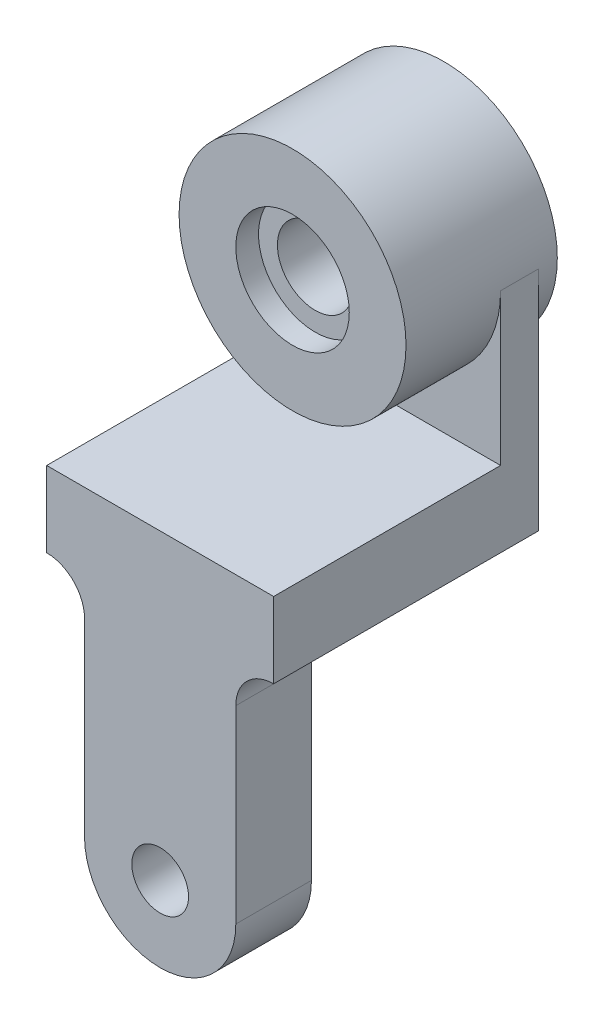
ISO-10303-21;
HEADER;
FILE_DESCRIPTION(('STEP AP214'),'2;1');
FILE_NAME('part.step','',(''),(''),'','','');
FILE_SCHEMA(('AUTOMOTIVE_DESIGN { 1 0 10303 214 1 1 1 1 }'));
ENDSEC;
DATA;
#1=APPLICATION_CONTEXT('core data for automotive mechanical design processes');
#2=APPLICATION_PROTOCOL_DEFINITION('international standard','automotive_design',2000,#1);
#3=PRODUCT_CONTEXT('',#1,'mechanical');
#4=PRODUCT('Part','Part','',(#3));
#5=PRODUCT_RELATED_PRODUCT_CATEGORY('part','',(#4));
#6=PRODUCT_DEFINITION_FORMATION('','',#4);
#7=PRODUCT_DEFINITION_CONTEXT('part definition',#1,'design');
#8=PRODUCT_DEFINITION('design','',#6,#7);
#9=PRODUCT_DEFINITION_SHAPE('','',#8);
#10=(LENGTH_UNIT() NAMED_UNIT(*) SI_UNIT(.MILLI.,.METRE.));
#11=(NAMED_UNIT(*) PLANE_ANGLE_UNIT() SI_UNIT($,.RADIAN.));
#12=(NAMED_UNIT(*) SI_UNIT($,.STERADIAN.) SOLID_ANGLE_UNIT());
#13=UNCERTAINTY_MEASURE_WITH_UNIT(LENGTH_MEASURE(1.E-05),#10,'distance_accuracy_value','');
#14=(GEOMETRIC_REPRESENTATION_CONTEXT(3) GLOBAL_UNCERTAINTY_ASSIGNED_CONTEXT((#13)) GLOBAL_UNIT_ASSIGNED_CONTEXT((#10,
#11,#12)) REPRESENTATION_CONTEXT('',''));
#15=CARTESIAN_POINT('',(0.,0.,0.));
#16=DIRECTION('',(0.,0.,1.));
#17=DIRECTION('',(1.,0.,0.));
#18=AXIS2_PLACEMENT_3D('',#15,#16,#17);
#19=CARTESIAN_POINT('',(0.,60.,-40.));
#20=DIRECTION('',(0.,0.,1.));
#21=DIRECTION('',(1.,0.,0.));
#22=AXIS2_PLACEMENT_3D('',#19,#20,#21);
#23=CYLINDRICAL_SURFACE('',#22,10.);
#24=CARTESIAN_POINT('',(0.,60.,-6.));
#25=DIRECTION('',(0.,0.,1.));
#26=DIRECTION('',(1.,0.,0.));
#27=AXIS2_PLACEMENT_3D('',#24,#25,#26);
#28=CIRCLE('',#27,10.);
#29=CARTESIAN_POINT('',(10.,60.,-6.));
#30=VERTEX_POINT('',#29);
#31=EDGE_CURVE('E212',#30,#30,#28,.F.);
#32=ORIENTED_EDGE('',*,*,#31,.F.);
#33=EDGE_LOOP('',(#32));
#34=FACE_BOUND('',#33,.T.);
#35=CARTESIAN_POINT('',(0.,60.,-34.));
#36=DIRECTION('',(0.,0.,-1.));
#37=DIRECTION('',(-1.,0.,0.));
#38=AXIS2_PLACEMENT_3D('',#35,#36,#37);
#39=CIRCLE('',#38,10.);
#40=CARTESIAN_POINT('',(-10.,60.,-34.));
#41=VERTEX_POINT('',#40);
#42=EDGE_CURVE('E216',#41,#41,#39,.F.);
#43=ORIENTED_EDGE('',*,*,#42,.F.);
#44=EDGE_LOOP('',(#43));
#45=FACE_BOUND('',#44,.T.);
#46=ADVANCED_FACE('F39',(#34,#45),#23,.F.);
#47=CARTESIAN_POINT('',(-30.,20.,35.));
#48=DIRECTION('',(0.,-1.,0.));
#49=DIRECTION('',(0.,0.,-1.));
#50=AXIS2_PLACEMENT_3D('',#47,#48,#49);
#51=PLANE('',#50);
#52=DIRECTION('',(1.,0.,0.));
#53=VECTOR('',#52,1.);
#54=CARTESIAN_POINT('',(-30.,20.,-25.));
#55=LINE('',#54,#53);
#56=CARTESIAN_POINT('',(-30.,20.,-25.));
#57=VERTEX_POINT('',#56);
#58=CARTESIAN_POINT('',(30.,20.,-25.));
#59=VERTEX_POINT('',#58);
#60=EDGE_CURVE('E126',#57,#59,#55,.T.);
#61=ORIENTED_EDGE('',*,*,#60,.F.);
#62=DIRECTION('',(0.,0.,-1.));
#63=VECTOR('',#62,1.);
#64=CARTESIAN_POINT('',(-30.,20.,35.));
#65=LINE('',#64,#63);
#66=CARTESIAN_POINT('',(-30.,20.,35.));
#67=VERTEX_POINT('',#66);
#68=EDGE_CURVE('E188',#67,#57,#65,.T.);
#69=ORIENTED_EDGE('',*,*,#68,.F.);
#70=DIRECTION('',(-1.,0.,0.));
#71=VECTOR('',#70,1.);
#72=CARTESIAN_POINT('',(-30.,20.,35.));
#73=LINE('',#72,#71);
#74=CARTESIAN_POINT('',(30.,20.,35.));
#75=VERTEX_POINT('',#74);
#76=EDGE_CURVE('E189',#75,#67,#73,.T.);
#77=ORIENTED_EDGE('',*,*,#76,.F.);
#78=DIRECTION('',(0.,0.,-1.));
#79=VECTOR('',#78,1.);
#80=CARTESIAN_POINT('',(30.,20.,35.));
#81=LINE('',#80,#79);
#82=EDGE_CURVE('E198',#75,#59,#81,.T.);
#83=ORIENTED_EDGE('',*,*,#82,.T.);
#84=EDGE_LOOP('',(#61,#69,#77,#83));
#85=FACE_BOUND('',#84,.T.);
#86=ADVANCED_FACE('F264',(#85),#51,.F.);
#87=CARTESIAN_POINT('',(-30.,0.,35.));
#88=DIRECTION('',(0.,1.,0.));
#89=DIRECTION('',(0.,0.,1.));
#90=AXIS2_PLACEMENT_3D('',#87,#88,#89);
#91=PLANE('',#90);
#92=DIRECTION('',(-1.,0.,0.));
#93=VECTOR('',#92,1.);
#94=CARTESIAN_POINT('',(-20.,0.,15.));
#95=LINE('',#94,#93);
#96=CARTESIAN_POINT('',(30.,0.,15.));
#97=VERTEX_POINT('',#96);
#98=CARTESIAN_POINT('',(-30.,0.,15.));
#99=VERTEX_POINT('',#98);
#100=EDGE_CURVE('E169',#97,#99,#95,.T.);
#101=ORIENTED_EDGE('',*,*,#100,.T.);
#102=DIRECTION('',(0.,0.,-1.));
#103=VECTOR('',#102,1.);
#104=CARTESIAN_POINT('',(-30.,0.,35.));
#105=LINE('',#104,#103);
#106=CARTESIAN_POINT('',(-30.,0.,-35.));
#107=VERTEX_POINT('',#106);
#108=EDGE_CURVE('E203',#99,#107,#105,.T.);
#109=ORIENTED_EDGE('',*,*,#108,.T.);
#110=DIRECTION('',(1.,0.,0.));
#111=VECTOR('',#110,1.);
#112=CARTESIAN_POINT('',(-30.,0.,-35.));
#113=LINE('',#112,#111);
#114=CARTESIAN_POINT('',(30.,0.,-35.));
#115=VERTEX_POINT('',#114);
#116=EDGE_CURVE('E194',#107,#115,#113,.T.);
#117=ORIENTED_EDGE('',*,*,#116,.T.);
#118=DIRECTION('',(0.,0.,-1.));
#119=VECTOR('',#118,1.);
#120=CARTESIAN_POINT('',(30.,0.,35.));
#121=LINE('',#120,#119);
#122=EDGE_CURVE('E202',#97,#115,#121,.T.);
#123=ORIENTED_EDGE('',*,*,#122,.F.);
#124=EDGE_LOOP('',(#101,#109,#117,#123));
#125=FACE_BOUND('',#124,.T.);
#126=ADVANCED_FACE('F260',(#125),#91,.F.);
#127=CARTESIAN_POINT('',(-30.,0.,35.));
#128=DIRECTION('',(1.,0.,0.));
#129=DIRECTION('',(0.,0.,-1.));
#130=AXIS2_PLACEMENT_3D('',#127,#128,#129);
#131=PLANE('',#130);
#132=DIRECTION('',(0.,-1.,0.));
#133=VECTOR('',#132,1.);
#134=CARTESIAN_POINT('',(-30.,0.,-35.));
#135=LINE('',#134,#133);
#136=CARTESIAN_POINT('',(-30.,60.,-35.));
#137=VERTEX_POINT('',#136);
#138=EDGE_CURVE('E179',#137,#107,#135,.T.);
#139=ORIENTED_EDGE('',*,*,#138,.T.);
#140=ORIENTED_EDGE('',*,*,#108,.F.);
#141=CARTESIAN_POINT('',(-30.,0.,35.));
#142=VERTEX_POINT('',#141);
#143=EDGE_CURVE('E207',#142,#99,#105,.T.);
#144=ORIENTED_EDGE('',*,*,#143,.F.);
#145=DIRECTION('',(0.,-1.,0.));
#146=VECTOR('',#145,1.);
#147=CARTESIAN_POINT('',(-30.,0.,35.));
#148=LINE('',#147,#146);
#149=EDGE_CURVE('E182',#67,#142,#148,.T.);
#150=ORIENTED_EDGE('',*,*,#149,.F.);
#151=ORIENTED_EDGE('',*,*,#68,.T.);
#152=DIRECTION('',(0.,1.,0.));
#153=VECTOR('',#152,1.);
#154=CARTESIAN_POINT('',(-30.,0.,-25.));
#155=LINE('',#154,#153);
#156=CARTESIAN_POINT('',(-30.,60.,-25.));
#157=VERTEX_POINT('',#156);
#158=EDGE_CURVE('E132',#57,#157,#155,.T.);
#159=ORIENTED_EDGE('',*,*,#158,.T.);
#160=DIRECTION('',(0.,0.,-1.));
#161=VECTOR('',#160,1.);
#162=CARTESIAN_POINT('',(-30.,60.,-25.));
#163=LINE('',#162,#161);
#164=EDGE_CURVE('E144',#157,#137,#163,.T.);
#165=ORIENTED_EDGE('',*,*,#164,.T.);
#166=EDGE_LOOP('',(#139,#140,#144,#150,#151,#159,#165));
#167=FACE_BOUND('',#166,.T.);
#168=ADVANCED_FACE('F251',(#167),#131,.F.);
#169=CARTESIAN_POINT('',(30.,0.,35.));
#170=DIRECTION('',(-1.,0.,0.));
#171=DIRECTION('',(0.,0.,1.));
#172=AXIS2_PLACEMENT_3D('',#169,#170,#171);
#173=PLANE('',#172);
#174=DIRECTION('',(0.,1.,0.));
#175=VECTOR('',#174,1.);
#176=CARTESIAN_POINT('',(30.,0.,-35.));
#177=LINE('',#176,#175);
#178=CARTESIAN_POINT('',(30.,60.,-35.));
#179=VERTEX_POINT('',#178);
#180=EDGE_CURVE('E136',#115,#179,#177,.T.);
#181=ORIENTED_EDGE('',*,*,#180,.T.);
#182=DIRECTION('',(0.,0.,-1.));
#183=VECTOR('',#182,1.);
#184=CARTESIAN_POINT('',(30.,60.,-25.));
#185=LINE('',#184,#183);
#186=CARTESIAN_POINT('',(30.,60.,-25.));
#187=VERTEX_POINT('',#186);
#188=EDGE_CURVE('E137',#187,#179,#185,.T.);
#189=ORIENTED_EDGE('',*,*,#188,.F.);
#190=DIRECTION('',(0.,-1.,0.));
#191=VECTOR('',#190,1.);
#192=CARTESIAN_POINT('',(30.,0.,-25.));
#193=LINE('',#192,#191);
#194=EDGE_CURVE('E125',#187,#59,#193,.T.);
#195=ORIENTED_EDGE('',*,*,#194,.T.);
#196=ORIENTED_EDGE('',*,*,#82,.F.);
#197=DIRECTION('',(0.,1.,0.));
#198=VECTOR('',#197,1.);
#199=CARTESIAN_POINT('',(30.,0.,35.));
#200=LINE('',#199,#198);
#201=CARTESIAN_POINT('',(30.,0.,35.));
#202=VERTEX_POINT('',#201);
#203=EDGE_CURVE('E187',#202,#75,#200,.T.);
#204=ORIENTED_EDGE('',*,*,#203,.F.);
#205=EDGE_CURVE('E205',#202,#97,#121,.T.);
#206=ORIENTED_EDGE('',*,*,#205,.T.);
#207=ORIENTED_EDGE('',*,*,#122,.T.);
#208=EDGE_LOOP('',(#181,#189,#195,#196,#204,#206,#207));
#209=FACE_BOUND('',#208,.T.);
#210=ADVANCED_FACE('F140',(#209),#173,.F.);
#211=CARTESIAN_POINT('',(0.,0.,35.));
#212=DIRECTION('',(0.,0.,-1.));
#213=DIRECTION('',(-1.,0.,0.));
#214=AXIS2_PLACEMENT_3D('',#211,#212,#213);
#215=PLANE('',#214);
#216=ORIENTED_EDGE('',*,*,#149,.T.);
#217=CARTESIAN_POINT('',(-30.,-10.,35.));
#218=DIRECTION('',(0.,0.,-1.));
#219=DIRECTION('',(-1.,0.,0.));
#220=AXIS2_PLACEMENT_3D('',#217,#218,#219);
#221=CIRCLE('',#220,10.);
#222=CARTESIAN_POINT('',(-20.,-10.,35.));
#223=VERTEX_POINT('',#222);
#224=EDGE_CURVE('E221',#142,#223,#221,.T.);
#225=ORIENTED_EDGE('',*,*,#224,.T.);
#226=DIRECTION('',(0.,-1.,0.));
#227=VECTOR('',#226,1.);
#228=CARTESIAN_POINT('',(-20.,0.,35.));
#229=LINE('',#228,#227);
#230=CARTESIAN_POINT('',(-20.,-60.,35.));
#231=VERTEX_POINT('',#230);
#232=EDGE_CURVE('E159',#223,#231,#229,.T.);
#233=ORIENTED_EDGE('',*,*,#232,.T.);
#234=CARTESIAN_POINT('',(0.,-60.,35.));
#235=DIRECTION('',(0.,0.,1.));
#236=DIRECTION('',(1.,0.,0.));
#237=AXIS2_PLACEMENT_3D('',#234,#235,#236);
#238=CIRCLE('',#237,20.);
#239=CARTESIAN_POINT('',(20.,-60.,35.));
#240=VERTEX_POINT('',#239);
#241=EDGE_CURVE('E173',#231,#240,#238,.T.);
#242=ORIENTED_EDGE('',*,*,#241,.T.);
#243=DIRECTION('',(0.,1.,0.));
#244=VECTOR('',#243,1.);
#245=CARTESIAN_POINT('',(20.,0.,35.));
#246=LINE('',#245,#244);
#247=CARTESIAN_POINT('',(20.,-10.,35.));
#248=VERTEX_POINT('',#247);
#249=EDGE_CURVE('E165',#240,#248,#246,.T.);
#250=ORIENTED_EDGE('',*,*,#249,.T.);
#251=CARTESIAN_POINT('',(30.,-10.,35.));
#252=DIRECTION('',(0.,0.,-1.));
#253=DIRECTION('',(-1.,0.,0.));
#254=AXIS2_PLACEMENT_3D('',#251,#252,#253);
#255=CIRCLE('',#254,10.);
#256=EDGE_CURVE('E50',#248,#202,#255,.T.);
#257=ORIENTED_EDGE('',*,*,#256,.T.);
#258=ORIENTED_EDGE('',*,*,#203,.T.);
#259=ORIENTED_EDGE('',*,*,#76,.T.);
#260=EDGE_LOOP('',(#216,#225,#233,#242,#250,#257,#258,#259));
#261=FACE_BOUND('',#260,.T.);
#262=CARTESIAN_POINT('',(0.,-60.,35.));
#263=DIRECTION('',(0.,0.,1.));
#264=DIRECTION('',(1.,0.,0.));
#265=AXIS2_PLACEMENT_3D('',#262,#263,#264);
#266=CIRCLE('',#265,7.5);
#267=CARTESIAN_POINT('',(7.5,-60.,35.));
#268=VERTEX_POINT('',#267);
#269=EDGE_CURVE('E141',#268,#268,#266,.T.);
#270=ORIENTED_EDGE('',*,*,#269,.F.);
#271=EDGE_LOOP('',(#270));
#272=FACE_BOUND('',#271,.T.);
#273=ADVANCED_FACE('F229',(#261,#272),#215,.F.);
#274=CARTESIAN_POINT('',(0.,0.,-35.));
#275=DIRECTION('',(0.,0.,-1.));
#276=DIRECTION('',(-1.,0.,0.));
#277=AXIS2_PLACEMENT_3D('',#274,#275,#276);
#278=PLANE('',#277);
#279=ORIENTED_EDGE('',*,*,#138,.F.);
#280=CARTESIAN_POINT('',(0.,60.,-35.));
#281=DIRECTION('',(0.,0.,1.));
#282=DIRECTION('',(-1.,0.,0.));
#283=AXIS2_PLACEMENT_3D('',#280,#281,#282);
#284=CIRCLE('',#283,30.);
#285=EDGE_CURVE('E134',#137,#179,#284,.T.);
#286=ORIENTED_EDGE('',*,*,#285,.T.);
#287=ORIENTED_EDGE('',*,*,#180,.F.);
#288=ORIENTED_EDGE('',*,*,#116,.F.);
#289=EDGE_LOOP('',(#279,#286,#287,#288));
#290=FACE_BOUND('',#289,.T.);
#291=ADVANCED_FACE('F258',(#290),#278,.T.);
#292=CARTESIAN_POINT('',(-20.,0.,15.));
#293=DIRECTION('',(-1.,0.,0.));
#294=DIRECTION('',(0.,-1.,0.));
#295=AXIS2_PLACEMENT_3D('',#292,#293,#294);
#296=PLANE('',#295);
#297=ORIENTED_EDGE('',*,*,#232,.F.);
#298=DIRECTION('',(0.,0.,1.));
#299=VECTOR('',#298,1.);
#300=CARTESIAN_POINT('',(-20.,-10.,15.));
#301=LINE('',#300,#299);
#302=CARTESIAN_POINT('',(-20.,-10.,15.));
#303=VERTEX_POINT('',#302);
#304=EDGE_CURVE('E208',#223,#303,#301,.F.);
#305=ORIENTED_EDGE('',*,*,#304,.T.);
#306=DIRECTION('',(0.,-1.,0.));
#307=VECTOR('',#306,1.);
#308=CARTESIAN_POINT('',(-20.,0.,15.));
#309=LINE('',#308,#307);
#310=CARTESIAN_POINT('',(-20.,-60.,15.));
#311=VERTEX_POINT('',#310);
#312=EDGE_CURVE('E163',#303,#311,#309,.T.);
#313=ORIENTED_EDGE('',*,*,#312,.T.);
#314=DIRECTION('',(0.,0.,1.));
#315=VECTOR('',#314,1.);
#316=CARTESIAN_POINT('',(-20.,-60.,15.));
#317=LINE('',#316,#315);
#318=EDGE_CURVE('E171',#311,#231,#317,.T.);
#319=ORIENTED_EDGE('',*,*,#318,.T.);
#320=EDGE_LOOP('',(#297,#305,#313,#319));
#321=FACE_BOUND('',#320,.T.);
#322=ADVANCED_FACE('F244',(#321),#296,.T.);
#323=CARTESIAN_POINT('',(20.,0.,15.));
#324=DIRECTION('',(1.,0.,0.));
#325=DIRECTION('',(0.,1.,0.));
#326=AXIS2_PLACEMENT_3D('',#323,#324,#325);
#327=PLANE('',#326);
#328=DIRECTION('',(0.,1.,0.));
#329=VECTOR('',#328,1.);
#330=CARTESIAN_POINT('',(20.,0.,15.));
#331=LINE('',#330,#329);
#332=CARTESIAN_POINT('',(20.,-60.,15.));
#333=VERTEX_POINT('',#332);
#334=CARTESIAN_POINT('',(20.,-10.,15.));
#335=VERTEX_POINT('',#334);
#336=EDGE_CURVE('E170',#333,#335,#331,.T.);
#337=ORIENTED_EDGE('',*,*,#336,.T.);
#338=DIRECTION('',(0.,0.,1.));
#339=VECTOR('',#338,1.);
#340=CARTESIAN_POINT('',(20.,-10.,15.));
#341=LINE('',#340,#339);
#342=EDGE_CURVE('E225',#335,#248,#341,.T.);
#343=ORIENTED_EDGE('',*,*,#342,.T.);
#344=ORIENTED_EDGE('',*,*,#249,.F.);
#345=DIRECTION('',(0.,0.,1.));
#346=VECTOR('',#345,1.);
#347=CARTESIAN_POINT('',(20.,-60.,15.));
#348=LINE('',#347,#346);
#349=EDGE_CURVE('E178',#333,#240,#348,.T.);
#350=ORIENTED_EDGE('',*,*,#349,.F.);
#351=EDGE_LOOP('',(#337,#343,#344,#350));
#352=FACE_BOUND('',#351,.T.);
#353=ADVANCED_FACE('F232',(#352),#327,.T.);
#354=CARTESIAN_POINT('',(0.,-60.,15.));
#355=DIRECTION('',(0.,0.,1.));
#356=DIRECTION('',(1.,0.,0.));
#357=AXIS2_PLACEMENT_3D('',#354,#355,#356);
#358=CYLINDRICAL_SURFACE('',#357,20.);
#359=ORIENTED_EDGE('',*,*,#241,.F.);
#360=ORIENTED_EDGE('',*,*,#318,.F.);
#361=CARTESIAN_POINT('',(0.,-60.,15.));
#362=DIRECTION('',(0.,0.,1.));
#363=DIRECTION('',(1.,0.,0.));
#364=AXIS2_PLACEMENT_3D('',#361,#362,#363);
#365=CIRCLE('',#364,20.);
#366=EDGE_CURVE('E161',#311,#333,#365,.T.);
#367=ORIENTED_EDGE('',*,*,#366,.T.);
#368=ORIENTED_EDGE('',*,*,#349,.T.);
#369=EDGE_LOOP('',(#359,#360,#367,#368));
#370=FACE_BOUND('',#369,.T.);
#371=ADVANCED_FACE('F245',(#370),#358,.T.);
#372=CARTESIAN_POINT('',(0.,-60.,15.));
#373=DIRECTION('',(0.,0.,1.));
#374=DIRECTION('',(1.,0.,0.));
#375=AXIS2_PLACEMENT_3D('',#372,#373,#374);
#376=PLANE('',#375);
#377=CARTESIAN_POINT('',(0.,-60.,15.));
#378=DIRECTION('',(0.,0.,1.));
#379=DIRECTION('',(1.,0.,0.));
#380=AXIS2_PLACEMENT_3D('',#377,#378,#379);
#381=CIRCLE('',#380,7.5);
#382=CARTESIAN_POINT('',(7.5,-60.,15.));
#383=VERTEX_POINT('',#382);
#384=EDGE_CURVE('E155',#383,#383,#381,.T.);
#385=ORIENTED_EDGE('',*,*,#384,.T.);
#386=EDGE_LOOP('',(#385));
#387=FACE_BOUND('',#386,.T.);
#388=ORIENTED_EDGE('',*,*,#312,.F.);
#389=CARTESIAN_POINT('',(-30.,-10.,15.));
#390=DIRECTION('',(0.,0.,1.));
#391=DIRECTION('',(1.,0.,0.));
#392=AXIS2_PLACEMENT_3D('',#389,#390,#391);
#393=CIRCLE('',#392,10.);
#394=EDGE_CURVE('E228',#303,#99,#393,.T.);
#395=ORIENTED_EDGE('',*,*,#394,.T.);
#396=ORIENTED_EDGE('',*,*,#100,.F.);
#397=CARTESIAN_POINT('',(30.,-10.,15.));
#398=DIRECTION('',(0.,0.,1.));
#399=DIRECTION('',(1.,0.,0.));
#400=AXIS2_PLACEMENT_3D('',#397,#398,#399);
#401=CIRCLE('',#400,10.);
#402=EDGE_CURVE('E11',#97,#335,#401,.T.);
#403=ORIENTED_EDGE('',*,*,#402,.T.);
#404=ORIENTED_EDGE('',*,*,#336,.F.);
#405=ORIENTED_EDGE('',*,*,#366,.F.);
#406=EDGE_LOOP('',(#388,#395,#396,#403,#404,#405));
#407=FACE_BOUND('',#406,.T.);
#408=ADVANCED_FACE('F238',(#387,#407),#376,.F.);
#409=CARTESIAN_POINT('',(0.,-60.,15.));
#410=DIRECTION('',(0.,0.,1.));
#411=DIRECTION('',(1.,0.,0.));
#412=AXIS2_PLACEMENT_3D('',#409,#410,#411);
#413=CYLINDRICAL_SURFACE('',#412,7.5);
#414=ORIENTED_EDGE('',*,*,#384,.F.);
#415=EDGE_LOOP('',(#414));
#416=FACE_BOUND('',#415,.T.);
#417=ORIENTED_EDGE('',*,*,#269,.T.);
#418=EDGE_LOOP('',(#417));
#419=FACE_BOUND('',#418,.T.);
#420=ADVANCED_FACE('F316',(#416,#419),#413,.F.);
#421=CARTESIAN_POINT('',(0.,60.,-25.));
#422=DIRECTION('',(0.,0.,-1.));
#423=DIRECTION('',(-1.,0.,0.));
#424=AXIS2_PLACEMENT_3D('',#421,#422,#423);
#425=PLANE('',#424);
#426=ORIENTED_EDGE('',*,*,#158,.F.);
#427=ORIENTED_EDGE('',*,*,#60,.T.);
#428=ORIENTED_EDGE('',*,*,#194,.F.);
#429=CARTESIAN_POINT('',(0.,60.,-25.));
#430=DIRECTION('',(0.,0.,1.));
#431=DIRECTION('',(-1.,0.,0.));
#432=AXIS2_PLACEMENT_3D('',#429,#430,#431);
#433=CIRCLE('',#432,30.);
#434=EDGE_CURVE('E130',#157,#187,#433,.T.);
#435=ORIENTED_EDGE('',*,*,#434,.F.);
#436=EDGE_LOOP('',(#426,#427,#428,#435));
#437=FACE_BOUND('',#436,.T.);
#438=ADVANCED_FACE('F123',(#437),#425,.F.);
#439=CARTESIAN_POINT('',(0.,60.,0.));
#440=DIRECTION('',(0.,0.,-1.));
#441=DIRECTION('',(-1.,0.,0.));
#442=AXIS2_PLACEMENT_3D('',#439,#440,#441);
#443=CYLINDRICAL_SURFACE('',#442,30.);
#444=ORIENTED_EDGE('',*,*,#188,.T.);
#445=ORIENTED_EDGE('',*,*,#285,.F.);
#446=ORIENTED_EDGE('',*,*,#164,.F.);
#447=ORIENTED_EDGE('',*,*,#434,.T.);
#448=EDGE_LOOP('',(#444,#445,#446,#447));
#449=FACE_BOUND('',#448,.T.);
#450=CARTESIAN_POINT('',(0.,60.,0.));
#451=DIRECTION('',(0.,0.,-1.));
#452=DIRECTION('',(-1.,0.,0.));
#453=AXIS2_PLACEMENT_3D('',#450,#451,#452);
#454=CIRCLE('',#453,30.);
#455=CARTESIAN_POINT('',(-30.,60.,0.));
#456=VERTEX_POINT('',#455);
#457=EDGE_CURVE('E154',#456,#456,#454,.T.);
#458=ORIENTED_EDGE('',*,*,#457,.T.);
#459=EDGE_LOOP('',(#458));
#460=FACE_BOUND('',#459,.T.);
#461=CARTESIAN_POINT('',(0.,60.,-40.));
#462=DIRECTION('',(0.,0.,-1.));
#463=DIRECTION('',(-1.,0.,0.));
#464=AXIS2_PLACEMENT_3D('',#461,#462,#463);
#465=CIRCLE('',#464,30.);
#466=CARTESIAN_POINT('',(-30.,60.,-40.));
#467=VERTEX_POINT('',#466);
#468=EDGE_CURVE('E211',#467,#467,#465,.T.);
#469=ORIENTED_EDGE('',*,*,#468,.F.);
#470=EDGE_LOOP('',(#469));
#471=FACE_BOUND('',#470,.T.);
#472=ADVANCED_FACE('F147',(#449,#460,#471),#443,.T.);
#473=CARTESIAN_POINT('',(0.,60.,0.));
#474=DIRECTION('',(0.,0.,-1.));
#475=DIRECTION('',(-1.,0.,0.));
#476=AXIS2_PLACEMENT_3D('',#473,#474,#475);
#477=PLANE('',#476);
#478=CARTESIAN_POINT('',(0.,60.,0.));
#479=DIRECTION('',(0.,0.,1.));
#480=DIRECTION('',(1.,0.,0.));
#481=AXIS2_PLACEMENT_3D('',#478,#479,#480);
#482=CIRCLE('',#481,15.);
#483=CARTESIAN_POINT('',(15.,60.,0.));
#484=VERTEX_POINT('',#483);
#485=EDGE_CURVE('E218',#484,#484,#482,.T.);
#486=ORIENTED_EDGE('',*,*,#485,.F.);
#487=EDGE_LOOP('',(#486));
#488=FACE_BOUND('',#487,.T.);
#489=ORIENTED_EDGE('',*,*,#457,.F.);
#490=EDGE_LOOP('',(#489));
#491=FACE_BOUND('',#490,.T.);
#492=ADVANCED_FACE('F309',(#488,#491),#477,.F.);
#493=CARTESIAN_POINT('',(0.,60.,-40.));
#494=DIRECTION('',(0.,0.,-1.));
#495=DIRECTION('',(-1.,0.,0.));
#496=AXIS2_PLACEMENT_3D('',#493,#494,#495);
#497=PLANE('',#496);
#498=CARTESIAN_POINT('',(0.,60.,-40.));
#499=DIRECTION('',(0.,0.,-1.));
#500=DIRECTION('',(-1.,0.,0.));
#501=AXIS2_PLACEMENT_3D('',#498,#499,#500);
#502=CIRCLE('',#501,15.);
#503=CARTESIAN_POINT('',(-15.,60.,-40.));
#504=VERTEX_POINT('',#503);
#505=EDGE_CURVE('E484',#504,#504,#502,.T.);
#506=ORIENTED_EDGE('',*,*,#505,.F.);
#507=EDGE_LOOP('',(#506));
#508=FACE_BOUND('',#507,.T.);
#509=ORIENTED_EDGE('',*,*,#468,.T.);
#510=EDGE_LOOP('',(#509));
#511=FACE_BOUND('',#510,.T.);
#512=ADVANCED_FACE('F303',(#508,#511),#497,.T.);
#513=CARTESIAN_POINT('',(0.,60.,-6.));
#514=DIRECTION('',(0.,0.,1.));
#515=DIRECTION('',(1.,0.,0.));
#516=AXIS2_PLACEMENT_3D('',#513,#514,#515);
#517=PLANE('',#516);
#518=CARTESIAN_POINT('',(0.,60.,-6.));
#519=DIRECTION('',(0.,0.,1.));
#520=DIRECTION('',(1.,0.,0.));
#521=AXIS2_PLACEMENT_3D('',#518,#519,#520);
#522=CIRCLE('',#521,15.);
#523=CARTESIAN_POINT('',(15.,60.,-6.));
#524=VERTEX_POINT('',#523);
#525=EDGE_CURVE('E213',#524,#524,#522,.T.);
#526=ORIENTED_EDGE('',*,*,#525,.T.);
#527=EDGE_LOOP('',(#526));
#528=FACE_BOUND('',#527,.T.);
#529=ORIENTED_EDGE('',*,*,#31,.T.);
#530=EDGE_LOOP('',(#529));
#531=FACE_BOUND('',#530,.T.);
#532=ADVANCED_FACE('F297',(#528,#531),#517,.T.);
#533=CARTESIAN_POINT('',(0.,60.,-6.));
#534=DIRECTION('',(0.,0.,1.));
#535=DIRECTION('',(1.,0.,0.));
#536=AXIS2_PLACEMENT_3D('',#533,#534,#535);
#537=CYLINDRICAL_SURFACE('',#536,15.);
#538=ORIENTED_EDGE('',*,*,#525,.F.);
#539=EDGE_LOOP('',(#538));
#540=FACE_BOUND('',#539,.T.);
#541=ORIENTED_EDGE('',*,*,#485,.T.);
#542=EDGE_LOOP('',(#541));
#543=FACE_BOUND('',#542,.T.);
#544=ADVANCED_FACE('F295',(#540,#543),#537,.F.);
#545=CARTESIAN_POINT('',(0.,60.,-34.));
#546=DIRECTION('',(0.,0.,-1.));
#547=DIRECTION('',(-1.,0.,0.));
#548=AXIS2_PLACEMENT_3D('',#545,#546,#547);
#549=PLANE('',#548);
#550=CARTESIAN_POINT('',(0.,60.,-34.));
#551=DIRECTION('',(0.,0.,-1.));
#552=DIRECTION('',(-1.,0.,0.));
#553=AXIS2_PLACEMENT_3D('',#550,#551,#552);
#554=CIRCLE('',#553,15.);
#555=CARTESIAN_POINT('',(-15.,60.,-34.));
#556=VERTEX_POINT('',#555);
#557=EDGE_CURVE('E220',#556,#556,#554,.T.);
#558=ORIENTED_EDGE('',*,*,#557,.T.);
#559=EDGE_LOOP('',(#558));
#560=FACE_BOUND('',#559,.T.);
#561=ORIENTED_EDGE('',*,*,#42,.T.);
#562=EDGE_LOOP('',(#561));
#563=FACE_BOUND('',#562,.T.);
#564=ADVANCED_FACE('F289',(#560,#563),#549,.T.);
#565=CARTESIAN_POINT('',(0.,60.,-34.));
#566=DIRECTION('',(0.,0.,-1.));
#567=DIRECTION('',(-1.,0.,0.));
#568=AXIS2_PLACEMENT_3D('',#565,#566,#567);
#569=CYLINDRICAL_SURFACE('',#568,15.);
#570=ORIENTED_EDGE('',*,*,#557,.F.);
#571=EDGE_LOOP('',(#570));
#572=FACE_BOUND('',#571,.T.);
#573=ORIENTED_EDGE('',*,*,#505,.T.);
#574=EDGE_LOOP('',(#573));
#575=FACE_BOUND('',#574,.T.);
#576=ADVANCED_FACE('F282',(#572,#575),#569,.F.);
#577=CARTESIAN_POINT('',(-30.,-10.,35.));
#578=DIRECTION('',(0.,0.,1.));
#579=DIRECTION('',(1.,0.,0.));
#580=AXIS2_PLACEMENT_3D('',#577,#578,#579);
#581=CYLINDRICAL_SURFACE('',#580,10.);
#582=ORIENTED_EDGE('',*,*,#394,.F.);
#583=ORIENTED_EDGE('',*,*,#304,.F.);
#584=ORIENTED_EDGE('',*,*,#224,.F.);
#585=ORIENTED_EDGE('',*,*,#143,.T.);
#586=EDGE_LOOP('',(#582,#583,#584,#585));
#587=FACE_BOUND('',#586,.T.);
#588=ADVANCED_FACE('F249',(#587),#581,.F.);
#589=CARTESIAN_POINT('',(30.,-10.,15.));
#590=DIRECTION('',(0.,0.,1.));
#591=DIRECTION('',(1.,0.,0.));
#592=AXIS2_PLACEMENT_3D('',#589,#590,#591);
#593=CYLINDRICAL_SURFACE('',#592,10.);
#594=ORIENTED_EDGE('',*,*,#402,.F.);
#595=ORIENTED_EDGE('',*,*,#205,.F.);
#596=ORIENTED_EDGE('',*,*,#256,.F.);
#597=ORIENTED_EDGE('',*,*,#342,.F.);
#598=EDGE_LOOP('',(#594,#595,#596,#597));
#599=FACE_BOUND('',#598,.T.);
#600=ADVANCED_FACE('F41',(#599),#593,.F.);
#601=CLOSED_SHELL('',(#46,#86,#126,#168,#210,#273,#291,#322,#353,#371,#408,#420,#438,#472,#492,
#512,#532,#544,#564,#576,#588,#600));
#602=MANIFOLD_SOLID_BREP('B2',#601);
#603=ADVANCED_BREP_SHAPE_REPRESENTATION('',(#18,#602),#14);
#604=SHAPE_DEFINITION_REPRESENTATION(#9,#603);
ENDSEC;
END-ISO-10303-21;
